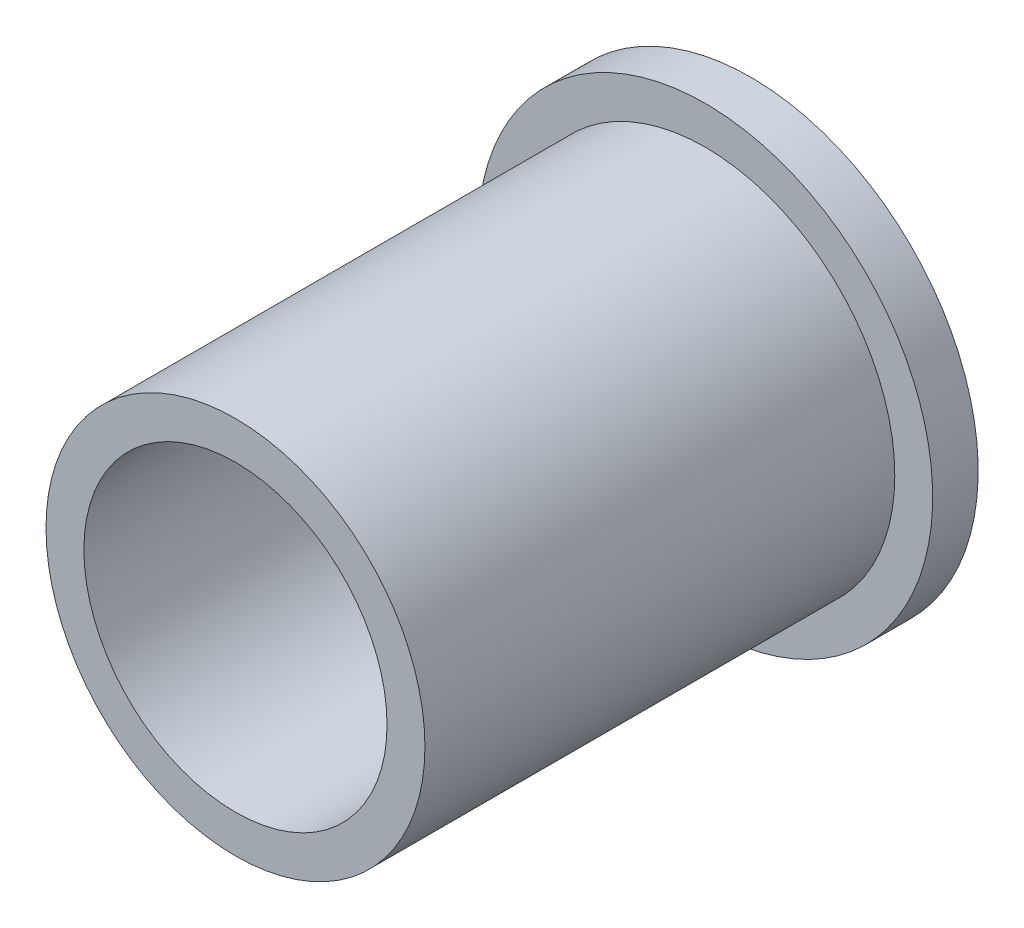
from build123d import *

# Parameters (mm, degrees)
BODY_PROFILE_25_R          = 12.5
BUSH_BODY_25X31_DEPTH      = 31
FLANGE_PROFILE_30_R        = 15
FLANGE_30X3_DEPTH          = 3
BORE_20_THROUGH_DEPTH      = 41.074929819
BORE_20_THROUGH_DEPTH_BACK = 41.074929819
BORE_PROFILE_20_R          = 10


with BuildPart() as part:
    # Body Profile Ø25 → Bush Body Ø25x31 (new body)
    with BuildSketch(Plane.XY):
        Circle(BODY_PROFILE_25_R)
    extrude(amount=BUSH_BODY_25X31_DEPTH)

    # Flange Profile Ø30 → Flange Ø30x3 (add)
    with BuildSketch(Plane(origin=(0, 0, 0), x_dir=(-1, 0, 0), z_dir=(0, 0, -1))):
        Circle(FLANGE_PROFILE_30_R)
    extrude(amount=FLANGE_30X3_DEPTH)

    # Bore Profile Ø20 → Bore Ø20 Through (cut, two sides: drawn at the far end of the back side and taken through both)
    with BuildSketch(Plane(origin=(0, 0, -3), x_dir=(-1, 0, 0), z_dir=(0, 0, -1)).offset(-BORE_20_THROUGH_DEPTH_BACK)):
        Circle(BORE_PROFILE_20_R)
    extrude(amount=BORE_20_THROUGH_DEPTH + BORE_20_THROUGH_DEPTH_BACK, mode=Mode.SUBTRACT)


solid = part.part
